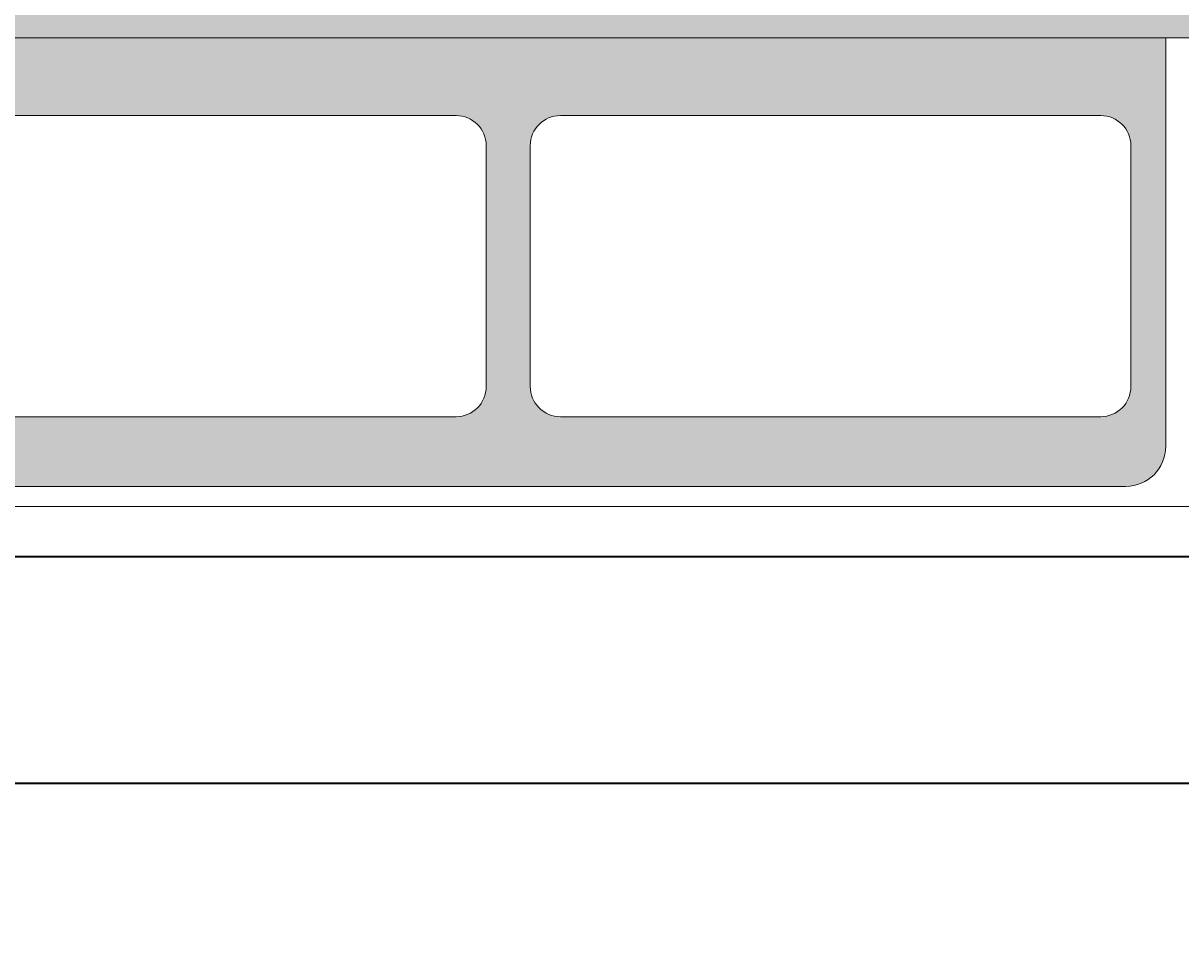
# Model space of a CAD drawing. Units: millimetres. Extents: x 27017497 to 27018854, y 7058029 to 7059154.
# Tile 74 of 91: x 27018390 to 27018436, y 7058126 to 7058163. Entities that reach past the tile are written whole.
import ezdxf

# ---------------------------------------------------------------- set-up
doc = ezdxf.new("R2010")
doc.units = ezdxf.units.MM
for name, color, linetype, lineweight in [('A-ANNO-DIMS', 2, 'Continuous', 18), ('A-FURN', 8, 'Continuous', 18), ('A-WALL', 7, 'Continuous', 35)]:
    doc.layers.add(name, color=color, linetype=linetype, lineweight=lineweight)
doc.layers.add('A-FURN-PATT', color=177, linetype='Continuous', lineweight=13, true_color=0x293189)
doc.styles.get("Standard").update_dxf_attribs({"font": 'arial.ttf'})
doc.dimstyles.get("Standard").update_dxf_attribs({"dimtxt": 0.18, "dimasz": 0.18, "dimexe": 0.18, "dimexo": 0.0625, "dimgap": 0.09, "dimtad": 0, "dimtih": 1, "dimtoh": 1, "dimdec": 4, "dimzin": 0, "dimdsep": 46, "dimtxsty": 'Standard', "dimcen": 0.09, "dimadec": 0, "dimazin": 0, "dimtfac": 1, "dimtdec": 4, "dimtofl": 0, "dimtmove": 0, "dimatfit": 3, "dimfxl": 1, "dimtolj": 1, "dimtzin": 0, "dimarcsym": 0})

# ---------------------------------------------------------------- blocks, each defined once
blk = doc.blocks.new('CAMMAT')
for p, q in [((1.2731, 0), (-1.2731, 0)), ((1.2731, -0.05), (-1.2731, -0.05)), ((0.61, -0.07), (-0.61, -0.07)), ((-0.65, -0.11), (-0.65, -0.5169)), ((-0.0465, -0.1395), (-0.5852, -0.1395)), ((0.5962, -0.1395), (0.0574, -0.1395)), ((-0.6152, -0.1695), (-0.6152, -0.4095)), ((-0.0165, -0.1695), (-0.0165, -0.4095)), ((0.0274, -0.1695), (0.0274, -0.4095)), ((-0.0465, -0.4395), (-0.5852, -0.4395)), ((0.5962, -0.4395), (0.0574, -0.4395)), ((-0.6904, -0.5169), (0.6826, -0.5169))]:
    blk.add_line(p, q)
for centre, radius, start, end in [((-0.61, -0.11), 0.04, 90, 180), ((-0.5852, -0.1695), 0.03, 90, 180), ((-0.0465, -0.1695), 0.03, 360, 90), ((0.0574, -0.1695), 0.03, 90, 180), ((-0.5852, -0.4095), 0.03, 180, 270), ((-0.0465, -0.4095), 0.03, 270, 360), ((0.0574, -0.4095), 0.03, 180, 270)]:
    blk.add_arc(centre, radius, start, end)
blk = doc.blocks.new('*D47')
at = {"layer": 'A-ANNO-DIMS', "color": 0, "lineweight": -2, "transparency": 16777216}
for p, q in [((27017561.166, 7058294.35), (27017561.166, 7058028.6)), ((27018790.606, 7058294.35), (27018790.606, 7058028.6)), ((27017561.346, 7058028.78), (27018175.431, 7058028.78)), ((27018790.426, 7058028.78), (27018176.341, 7058028.78))]:
    blk.add_line(p, q, dxfattribs=at)
at = {"layer": 'A-ANNO-DIMS', "color": 0, "transparency": 16777216}
for points in [[(27017561.346, 7058028.81), (27017561.346, 7058028.75), (27017561.166, 7058028.78)], [(27018790.426, 7058028.81), (27018790.426, 7058028.75), (27018790.606, 7058028.78)]]:
    blk.add_solid(points, dxfattribs=at)
at = {"layer": 'Defpoints', "color": 0, "transparency": 16777216}
for p in [(27017561.166, 7058294.412), (27018790.606, 7058294.412), (27018790.606, 7058028.78)]:
    blk.add_point(p, dxfattribs=at)
at = {"layer": 'A-ANNO-DIMS', "color": 0, "transparency": 16777216, "insert": (27018175.886, 7058028.78), "char_height": 0.18, "attachment_point": 5}
blk.add_mtext('\\A1;1229.4', dxfattribs=at)
blk = doc.blocks.new('*D48')
at = {"layer": 'A-ANNO-DIMS', "color": 0, "lineweight": -2, "transparency": 16777216}
for p, q in [((27018463.498, 7058622.912), (27017497.536, 7058622.912)), ((27017497.716, 7058622.732), (27017497.716, 7058357.753)), ((27017497.716, 7058092.41), (27017497.716, 7058357.389)), ((27018555.129, 7058092.23), (27017497.536, 7058092.23))]:
    blk.add_line(p, q, dxfattribs=at)
at = {"layer": 'A-ANNO-DIMS', "color": 0, "transparency": 16777216}
for points in [[(27017497.686, 7058622.732), (27017497.746, 7058622.732), (27017497.716, 7058622.912)], [(27017497.686, 7058092.41), (27017497.746, 7058092.41), (27017497.716, 7058092.23)]]:
    blk.add_solid(points, dxfattribs=at)
at = {"layer": 'Defpoints', "color": 0, "transparency": 16777216}
for p in [(27018463.561, 7058622.912), (27017497.716, 7058092.23), (27018555.192, 7058092.23)]:
    blk.add_point(p, dxfattribs=at)
at = {"layer": 'A-ANNO-DIMS', "color": 0, "transparency": 16777216, "insert": (27017497.716, 7058357.571), "char_height": 0.18, "attachment_point": 5}
blk.add_mtext('\\A1;530.7', dxfattribs=at)

msp = doc.modelspace()

# ---------------------------------------------------------------- hatches: boundary and pattern name
at = {"layer": 'A-FURN-PATT'}
h = msp.add_hatch(color=256, dxfattribs=at)
h.dxf.hatch_style = 1
h.paths.add_polyline_path([(27018435.86, 7058218.784, 0.414214), (27018434.267, 7058220.377), (27018385.674, 7058220.377, 0.414214), (27018384.081, 7058218.784), (27018384.081, 7058174.59), (27018387.977, 7058174.891), (27018391.56, 7058175.393), (27018394.078, 7058176.128), (27018395.791, 7058177.21), (27018396.958, 7058178.748), (27018397.838, 7058180.854), (27018398.69, 7058183.639), (27018399.293, 7058180.835), (27018399.836, 7058178.594), (27018400.426, 7058176.691), (27018401.17, 7058174.899), (27018402.177, 7058172.991), (27018403.552, 7058170.741), (27018405.403, 7058167.922), (27018407.838, 7058164.308), (27018410.273, 7058167.922), (27018412.124, 7058170.741), (27018413.499, 7058172.991), (27018414.506, 7058174.899), (27018415.25, 7058176.691), (27018415.84, 7058178.594), (27018416.383, 7058180.835), (27018416.986, 7058183.639), (27018417.838, 7058180.854), (27018418.718, 7058178.748), (27018419.885, 7058177.21), (27018421.598, 7058176.128), (27018424.116, 7058175.393), (27018427.699, 7058174.891), (27018432.604, 7058174.513), (27018435.86, 7058174.329)])
h.paths.add_polyline_path([(27018439.093, 7058174.146), (27018432.604, 7058174.513), (27018427.699, 7058174.891), (27018424.116, 7058175.393), (27018421.598, 7058176.128), (27018419.885, 7058177.21), (27018418.718, 7058178.748), (27018417.838, 7058180.854), (27018416.986, 7058183.639), (27018416.383, 7058180.835), (27018415.84, 7058178.594), (27018415.25, 7058176.691), (27018414.506, 7058174.899), (27018413.499, 7058172.991), (27018412.124, 7058170.741), (27018410.273, 7058167.922), (27018407.838, 7058164.308)])
h.paths.add_polyline_path([(27018403.552, 7058170.741), (27018402.177, 7058172.991), (27018401.17, 7058174.899), (27018400.426, 7058176.691), (27018399.836, 7058178.594), (27018399.293, 7058180.835), (27018398.69, 7058183.639), (27018397.838, 7058180.854), (27018396.958, 7058178.748), (27018395.791, 7058177.21), (27018394.078, 7058176.128), (27018391.56, 7058175.393), (27018387.977, 7058174.891), (27018383.071, 7058174.513), (27018376.583, 7058174.146), (27018407.838, 7058164.308), (27018405.403, 7058167.922)])
h.paths.add_polyline_path([(27018437.469, 7058173.635), (27018407.838, 7058164.308), (27018382.784, 7058172.194), (27018382.784, 7058162.502), (27018437.469, 7058162.502)])
h.paths.add_polyline_path([(27018435.86, 7058162.502), (27018384.081, 7058162.502), (27018384.081, 7058146.294, 0.414214), (27018385.674, 7058144.7), (27018434.267, 7058144.7, 0.414214), (27018435.86, 7058146.294)])
h.paths.add_polyline_path([(27018407.684, 7058159.418, -0.41419), (27018408.879, 7058158.223), (27018408.879, 7058148.664, -0.414237), (27018407.684, 7058147.469), (27018386.224, 7058147.469, -0.41419), (27018385.029, 7058148.663), (27018385.029, 7058158.223, -0.414237), (27018386.224, 7058159.418)], flags=16)
h.paths.add_polyline_path([(27018411.821, 7058159.418), (27018433.28, 7058159.418, -0.41419), (27018434.475, 7058158.223), (27018434.475, 7058148.664, -0.414237), (27018433.28, 7058147.469), (27018411.821, 7058147.469, -0.414214), (27018410.626, 7058148.664), (27018410.626, 7058158.223, -0.414214)], flags=16)
h.paths.add_polyline_path([(27018382.886, 7058160.632), (27018362.971, 7058160.632), (27018362.971, 7058144.7), (27018382.886, 7058144.7)])
h.paths.add_polyline_path([(27018379.136, 7058152.033, -1), (27018367.187, 7058152.033, -1)], flags=16)
h.paths.add_polyline_path([(27018376.861, 7058152.033, -1), (27018369.461, 7058152.033, -1)], flags=0)
h.paths.add_polyline_path([(27018456.97, 7058160.632), (27018437.055, 7058160.632), (27018437.055, 7058144.7), (27018456.97, 7058144.7)])
h.paths.add_polyline_path([(27018453.028, 7058152.033, -1), (27018441.079, 7058152.033, -1)], flags=16)
h.paths.add_polyline_path([(27018450.754, 7058152.033, -1), (27018443.354, 7058152.033, -1)], flags=0)
h.paths.add_polyline_path([(27018434.475, 7058158.223, 0.41419), (27018433.28, 7058159.418), (27018411.821, 7058159.418, 0.414214), (27018410.626, 7058158.223), (27018410.626, 7058148.664, 0.414214), (27018411.821, 7058147.469), (27018433.28, 7058147.469, 0.414237), (27018434.475, 7058148.664)], flags=0)

# ---------------------------------------------------------------- linework, layer by layer
at = {"layer": 'A-WALL'}
for p, q in [((27018468.106, 7058141.912), (27018319.606, 7058141.912)), ((27018468.106, 7058132.912), (27018310.606, 7058132.912))]:
    msp.add_line(p, q, dxfattribs=at)

# ---------------------------------------------------------------- block references
at = {"layer": 'A-FURN', "xscale": 39.82996475819422, "yscale": 39.82996475819422, "zscale": 39.82996475819422, "rotation": 180}
msp.add_blockref('CAMMAT', (27018409.97, 7058141.912), dxfattribs=at)

# ---------------------------------------------------------------- dimensions: what is measured, and where the dimension line sits
at = {"layer": 'A-ANNO-DIMS'}
dim = msp.add_linear_dim(base=(27017497.716, 7058092.23), p1=(27018463.561, 7058622.912), p2=(27018555.192, 7058092.23), angle=90, dimstyle='Standard', override={"dimdec": 1, "dimlfac": 1, "dimrnd": 0, "dimzin": 0, "dimdsep": 46, "dimlunit": 2}, dxfattribs=at)
dim.commit()
dim.dimension.update_dxf_attribs({"geometry": '*D48', "text_midpoint": (27017497.716, 7058357.571)})
dim = msp.add_linear_dim(base=(27018790.606, 7058028.78), p1=(27017561.166, 7058294.412), p2=(27018790.606, 7058294.412), dimstyle='Standard', override={"dimdec": 1, "dimlfac": 1, "dimrnd": 0, "dimzin": 0, "dimdsep": 46, "dimlunit": 2}, dxfattribs=at)
dim.commit()
dim.dimension.update_dxf_attribs({"geometry": '*D47', "text_midpoint": (27018175.886, 7058028.78)})

doc.saveas('drawing.dxf')
